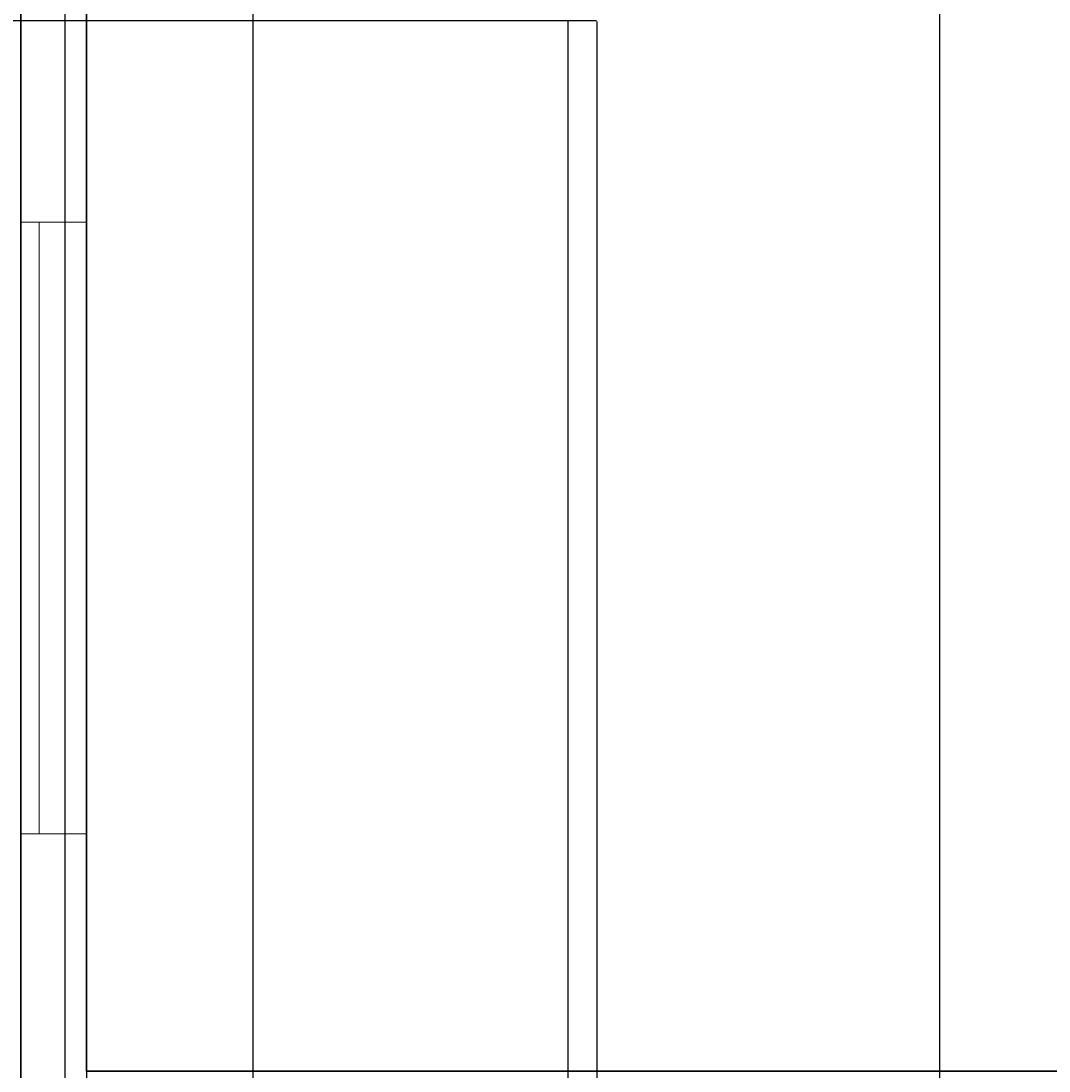
# Model space of a CAD drawing. Units: inches. Extents: x 867 to 1667, y -234 to 788.
# Tile 11 of 42: x 1071 to 1212, y -8 to 136. Entities that reach past the tile are written whole.
import ezdxf

# ---------------------------------------------------------------- set-up
doc = ezdxf.new("R2010")
doc.units = ezdxf.units.IN
doc.header["$MEASUREMENT"] = 0
for name, color, linetype, lineweight in [('A-ANNO-DIMS', 2, 'Continuous', 18), ('A-Glaz', 92, 'Continuous', 18), ('A-Wall', 7, 'Continuous', 35)]:
    doc.layers.add(name, color=color, linetype=linetype, lineweight=lineweight)
doc.styles.get("Standard").update_dxf_attribs({"font": 'arial.ttf'})
doc.dimstyles.get("Standard").update_dxf_attribs({"dimtxt": 0.6875, "dimasz": 0.18, "dimexe": 0.18, "dimexo": 0.0625, "dimgap": 0.09, "dimtad": 0, "dimdec": 4, "dimzin": 0, "dimdsep": 46, "dimlunit": 4, "dimtxsty": 'Standard', "dimcen": 0.09, "dimadec": 0, "dimazin": 0, "dimtfac": 1, "dimtdec": 4, "dimtofl": 0, "dimtmove": 0, "dimatfit": 3, "dimfxl": 1, "dimtolj": 1, "dimtzin": 0, "dimarcsym": 0})

# ---------------------------------------------------------------- blocks, each defined once
blk = doc.blocks.new('WIN-83_90IN')
for p, q in [((0, 83.9), (9, 83.9)), ((2.51, 83.9), (2.51, 0)), ((6.08, 0), (6.08, 83.9)), ((0, 0), (9, 0))]:
    blk.add_line(p, q)
blk = doc.blocks.new('*D29')
at = {"layer": 'A-ANNO-DIMS', "color": 0, "lineweight": -2, "transparency": 16777216}
for p, q in [((1076.89, 623.55), (1076.89, -233.54)), ((1102.67, 623.55), (1102.67, -233.54)), ((1077.07, -233.36), (1088.52, -233.36)), ((1102.49, -233.36), (1091.03, -233.36))]:
    blk.add_line(p, q, dxfattribs=at)
at = {"layer": 'A-ANNO-DIMS', "color": 0, "transparency": 16777216}
for points in [[(1077.07, -233.33), (1077.07, -233.39), (1076.89, -233.36)], [(1102.49, -233.33), (1102.49, -233.39), (1102.67, -233.36)]]:
    blk.add_solid(points, dxfattribs=at)
at = {"layer": 'Defpoints', "color": 0, "transparency": 16777216}
for p in [(1076.89, 623.62), (1102.67, 623.62), (1102.67, -233.36)]:
    blk.add_point(p, dxfattribs=at)
at = {"layer": 'A-ANNO-DIMS', "color": 0, "transparency": 16777216, "insert": (1089.78, -233.36), "char_height": 0.688, "attachment_point": 5}
blk.add_mtext('\\A1;25.78', dxfattribs=at)
blk = doc.blocks.new('*D37')
at = {"layer": 'A-ANNO-DIMS', "color": 0, "lineweight": -2, "transparency": 16777216}
for p, q in [((1049.89, 257.55), (1049.89, -233.54)), ((1196.89, 257.55), (1196.89, -233.54)), ((1050.07, -233.36), (1122.57, -233.36)), ((1196.71, -233.36), (1124.2, -233.36))]:
    blk.add_line(p, q, dxfattribs=at)
at = {"layer": 'A-ANNO-DIMS', "color": 0, "transparency": 16777216}
for points in [[(1050.07, -233.33), (1050.07, -233.39), (1049.89, -233.36)], [(1196.71, -233.33), (1196.71, -233.39), (1196.89, -233.36)]]:
    blk.add_solid(points, dxfattribs=at)
at = {"layer": 'Defpoints', "color": 0, "transparency": 16777216}
for p in [(1049.89, 257.62), (1196.89, 257.62), (1196.89, -233.36)]:
    blk.add_point(p, dxfattribs=at)
at = {"layer": 'A-ANNO-DIMS', "color": 0, "transparency": 16777216, "insert": (1123.39, -233.36), "char_height": 0.688, "attachment_point": 5}
blk.add_mtext('\\A1;147', dxfattribs=at)
blk = doc.blocks.new('*D41')
at = {"layer": 'A-ANNO-DIMS', "color": 0, "lineweight": -2, "transparency": 16777216}
for p, q in [((1149.82, 221.62), (867.76, 221.62)), ((867.94, 221.44), (867.94, 179.85)), ((867.94, 136.3), (867.94, 177.88)), ((1149.82, 136.12), (867.76, 136.12))]:
    blk.add_line(p, q, dxfattribs=at)
at = {"layer": 'A-ANNO-DIMS', "color": 0, "transparency": 16777216}
for points in [[(867.91, 221.44), (867.97, 221.44), (867.94, 221.62)], [(867.91, 136.3), (867.97, 136.3), (867.94, 136.12)]]:
    blk.add_solid(points, dxfattribs=at)
at = {"layer": 'Defpoints', "color": 0, "transparency": 16777216}
for p in [(867.94, 221.62), (1149.89, 221.62), (1149.89, 136.12)]:
    blk.add_point(p, dxfattribs=at)
at = {"layer": 'A-ANNO-DIMS', "color": 0, "transparency": 16777216, "insert": (867.94, 178.87), "char_height": 0.688, "attachment_point": 5, "rotation": 90}
blk.add_mtext('\\A1;85.5', dxfattribs=at)
blk = doc.blocks.new('*D42')
at = {"layer": 'A-ANNO-DIMS', "color": 0, "lineweight": -2, "transparency": 16777216}
for p, q in [((1079.89, 136.05), (1079.89, -233.54)), ((1145.89, 136.05), (1145.89, -233.54)), ((1080.07, -233.36), (1112.3, -233.36)), ((1145.71, -233.36), (1113.47, -233.36))]:
    blk.add_line(p, q, dxfattribs=at)
at = {"layer": 'A-ANNO-DIMS', "color": 0, "transparency": 16777216}
for points in [[(1080.07, -233.33), (1080.07, -233.39), (1079.89, -233.36)], [(1145.71, -233.33), (1145.71, -233.39), (1145.89, -233.36)]]:
    blk.add_solid(points, dxfattribs=at)
at = {"layer": 'Defpoints', "color": 0, "transparency": 16777216}
for p in [(1079.89, 136.12), (1145.89, 136.12), (1145.89, -233.36)]:
    blk.add_point(p, dxfattribs=at)
at = {"layer": 'A-ANNO-DIMS', "color": 0, "transparency": 16777216, "insert": (1112.89, -233.36), "char_height": 0.688, "attachment_point": 5}
blk.add_mtext('\\A1;66', dxfattribs=at)
blk = doc.blocks.new('*D43')
at = {"layer": 'A-ANNO-DIMS', "color": 0, "lineweight": -2, "transparency": 16777216}
for p, q in [((1145.89, 136.05), (1145.89, -233.54)), ((1149.89, 136.05), (1149.89, -233.54)), ((1146.07, -233.36), (1147.56, -233.36)), ((1149.71, -233.36), (1148.21, -233.36))]:
    blk.add_line(p, q, dxfattribs=at)
at = {"layer": 'A-ANNO-DIMS', "color": 0, "transparency": 16777216}
for points in [[(1146.07, -233.33), (1146.07, -233.39), (1145.89, -233.36)], [(1149.71, -233.33), (1149.71, -233.39), (1149.89, -233.36)]]:
    blk.add_solid(points, dxfattribs=at)
at = {"layer": 'Defpoints', "color": 0, "transparency": 16777216}
for p in [(1145.89, 136.12), (1149.89, 136.12), (1149.89, -233.36)]:
    blk.add_point(p, dxfattribs=at)
at = {"layer": 'A-ANNO-DIMS', "color": 0, "transparency": 16777216, "insert": (1147.89, -233.36), "char_height": 0.688, "attachment_point": 5}
blk.add_mtext('\\A1;4', dxfattribs=at)

msp = doc.modelspace()

# ---------------------------------------------------------------- linework, layer by layer
at = {"layer": 'A-Wall'}
for p, q in [((1070.8866, 221.617), (1070.8866, -55.9081)), ((1079.8866, 221.617), (1079.8866, -7.883)), ((1247.8866, -7.883), (1079.8866, -7.883))]:
    msp.add_line(p, q, dxfattribs=at)

# ---------------------------------------------------------------- block references
at = {"layer": 'A-Glaz'}
msp.add_blockref('WIN-83_90IN', (1070.887, 24.651), dxfattribs=at)

# ---------------------------------------------------------------- dimensions: what is measured, and where the dimension line sits
at = {"layer": 'A-ANNO-DIMS'}
for base, p1, p2, override, picture, middle in [((1102.6661, -233.3581), (1076.8866, 623.617), (1102.6661, 623.617), {"dimdec": 2, "dimlfac": 1, "dimrnd": 0, "dimzin": 0, "dimdsep": 46, "dimlunit": 2}, '*D29', (1089.7763, -233.3581)), ((1196.8866, -233.3581), (1049.8866, 257.617), (1196.8866, 257.617), {"dimdec": 0, "dimlfac": 1, "dimrnd": 0, "dimzin": 0, "dimdsep": 46, "dimlunit": 2}, '*D37', (1123.3866, -233.3581)), ((1145.8866, -233.3581), (1079.8866, 136.117), (1145.8866, 136.117), {"dimdec": 0, "dimlfac": 1, "dimrnd": 0, "dimzin": 0, "dimdsep": 46, "dimlunit": 2}, '*D42', (1112.8866, -233.3581)), ((1149.8866, -233.3581), (1145.8866, 136.117), (1149.8866, 136.117), {"dimdec": 0, "dimlfac": 1, "dimrnd": 0, "dimzin": 0, "dimdsep": 46, "dimlunit": 2}, '*D43', (1147.8866, -233.3581))]:
    dim = msp.add_linear_dim(base=base, p1=p1, p2=p2, dimstyle='Standard', override=override, dxfattribs=at)
    dim.commit()
    dim.dimension.update_dxf_attribs({"geometry": picture, "text_midpoint": middle})
dim = msp.add_linear_dim(base=(867.9366, 221.617), p1=(1149.8866, 136.117), p2=(1149.8866, 221.617), angle=90, dimstyle='Standard', override={"dimdec": 1, "dimlfac": 1, "dimrnd": 0, "dimzin": 0, "dimdsep": 46, "dimlunit": 2}, dxfattribs=at)
dim.commit()
dim.dimension.update_dxf_attribs({"geometry": '*D41', "text_midpoint": (867.9366, 178.867)})

doc.saveas('drawing.dxf')
